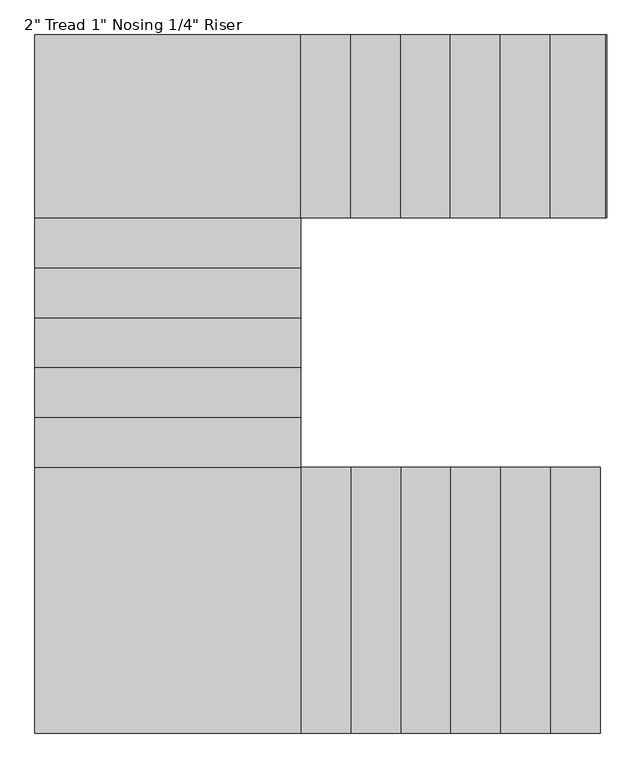
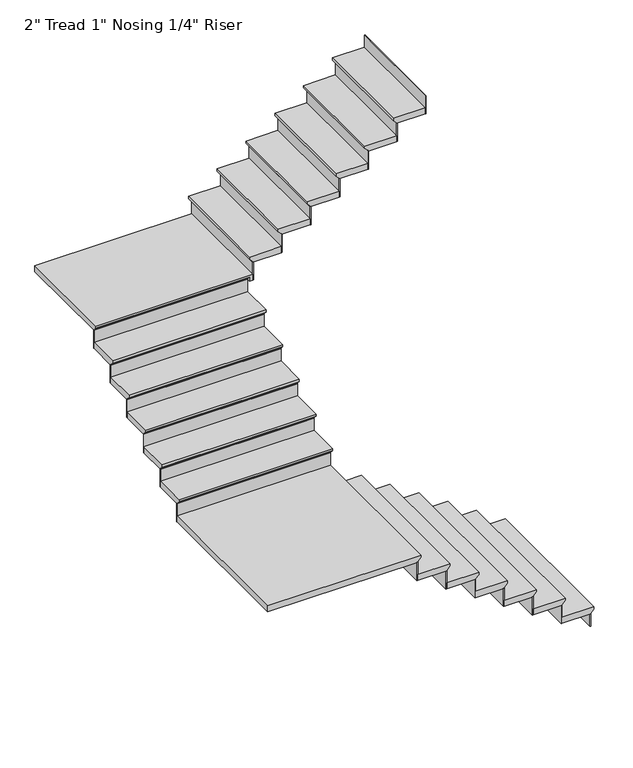
"""IFC4 building model written with IfcOpenShell, lengths in millimetres: stair flight geometry."""

from ifc_helpers import new_model, si_unit, origin, place, context, project, spatial, faceted_brep, source, transform, mapped, element, save


def stair_flight_e1114729(model_context):
    return source(origin(), model_context, "Body", "Brep", [
        faceted_brep([(-2515.2117403, -5163.0426559, 12782.55), (-2515.2117403, -5163.0426559, 12801.6), (-2515.2117403, -6382.2426559, 12801.6), (-2515.2117403, -6382.2426559, 12782.55), (-2540.6117403, -5163.0426559, 12757.15), (-2540.6117403, -6382.2426559, 12757.15), (-2769.2117403, -5163.0426559, 12801.6), (-2769.2117403, -6382.2426559, 12801.6), (-2540.6117403, -6382.2426559, 12750.8), (-2769.2117403, -6382.2426559, 12750.8), (-2769.2117403, -5163.0426559, 12750.8), (-2540.6117403, -5163.0426559, 12750.8)], [[[0, 1, 2, 3]], [[4, 0, 3, 5]], [[2, 1, 6, 7]], [[8, 9, 10, 11]], [[2, 7, 9, 8, 5, 3]], [[8, 11, 4, 5]], [[6, 1, 0, 4, 11, 10]], [[7, 6, 10, 9]]]),
        faceted_brep([(-2540.6117403, -5163.0426559, 12750.8), (-2540.6117403, -5163.0426559, 12649.2), (-2546.9617403, -5163.0426559, 12649.2), (-2546.9617403, -5163.0426559, 12750.8), (-2540.6117403, -6382.2426559, 12750.8), (-2546.9617403, -6382.2426559, 12750.8), (-2546.9617403, -6382.2426559, 12649.2), (-2540.6117403, -6382.2426559, 12649.2)], [[[0, 1, 2, 3]], [[4, 5, 6, 7]], [[1, 0, 4, 7]], [[2, 1, 7, 6]], [[3, 2, 6, 5]], [[0, 3, 5, 4]]]),
        faceted_brep([(-2769.2117403, -5163.0426559, 12903.2), (-2769.2117403, -5163.0426559, 12750.8), (-2775.5617403, -5163.0426559, 12750.8), (-2775.5617403, -5163.0426559, 12903.2), (-2769.2117403, -6382.2426559, 12903.2), (-2775.5617403, -6382.2426559, 12903.2), (-2775.5617403, -6382.2426559, 12750.8), (-2769.2117403, -6382.2426559, 12750.8)], [[[0, 1, 2, 3]], [[4, 5, 6, 7]], [[1, 0, 4, 7]], [[2, 1, 7, 6]], [[3, 2, 6, 5]], [[0, 3, 5, 4]]]),
        faceted_brep([(-2743.8117403, -6382.2426559, 12954.0), (-2743.8117403, -5163.0426559, 12954.0), (-2997.8117403, -5163.0426559, 12954.0), (-2997.8117403, -6382.2426559, 12954.0), (-2769.2117403, -6382.2426559, 12903.2), (-2997.8117403, -6382.2426559, 12903.2), (-2997.8117403, -5163.0426559, 12903.2), (-2769.2117403, -5163.0426559, 12903.2), (-2769.2117403, -6382.2426559, 12909.55), (-2743.8117403, -6382.2426559, 12934.95), (-2769.2117403, -5163.0426559, 12909.55), (-2743.8117403, -5163.0426559, 12934.95)], [[[0, 1, 2, 3]], [[4, 5, 6, 7]], [[0, 3, 5, 4, 8, 9]], [[4, 7, 10, 8]], [[2, 1, 11, 10, 7, 6]], [[3, 2, 6, 5]], [[11, 1, 0, 9]], [[10, 11, 9, 8]]]),
        faceted_brep([(-2997.8117403, -5163.0426559, 13055.6), (-2997.8117403, -5163.0426559, 12903.2), (-3004.1617403, -5163.0426559, 12903.2), (-3004.1617403, -5163.0426559, 13055.6), (-2997.8117403, -6382.2426559, 13055.6), (-3004.1617403, -6382.2426559, 13055.6), (-3004.1617403, -6382.2426559, 12903.2), (-2997.8117403, -6382.2426559, 12903.2)], [[[0, 1, 2, 3]], [[4, 5, 6, 7]], [[1, 0, 4, 7]], [[2, 1, 7, 6]], [[3, 2, 6, 5]], [[0, 3, 5, 4]]]),
        faceted_brep([(-2972.4117403, -6382.2426559, 13106.4), (-2972.4117403, -5163.0426559, 13106.4), (-3226.4117403, -5163.0426559, 13106.4), (-3226.4117403, -6382.2426559, 13106.4), (-2997.8117403, -6382.2426559, 13055.6), (-3226.4117403, -6382.2426559, 13055.6), (-3226.4117403, -5163.0426559, 13055.6), (-2997.8117403, -5163.0426559, 13055.6), (-2997.8117403, -6382.2426559, 13061.95), (-2972.4117403, -6382.2426559, 13087.35), (-2997.8117403, -5163.0426559, 13061.95), (-2972.4117403, -5163.0426559, 13087.35)], [[[0, 1, 2, 3]], [[4, 5, 6, 7]], [[0, 3, 5, 4, 8, 9]], [[4, 7, 10, 8]], [[2, 1, 11, 10, 7, 6]], [[3, 2, 6, 5]], [[11, 1, 0, 9]], [[10, 11, 9, 8]]]),
        faceted_brep([(-3226.4117403, -5163.0426559, 13208.0), (-3226.4117403, -5163.0426559, 13055.6), (-3232.7617403, -5163.0426559, 13055.6), (-3232.7617403, -5163.0426559, 13208.0), (-3226.4117403, -6382.2426559, 13208.0), (-3232.7617403, -6382.2426559, 13208.0), (-3232.7617403, -6382.2426559, 13055.6), (-3226.4117403, -6382.2426559, 13055.6)], [[[0, 1, 2, 3]], [[4, 5, 6, 7]], [[1, 0, 4, 7]], [[2, 1, 7, 6]], [[3, 2, 6, 5]], [[0, 3, 5, 4]]]),
        faceted_brep([(-3201.0117403, -6382.2426559, 13258.8), (-3201.0117403, -5163.0426559, 13258.8), (-3455.0117403, -5163.0426559, 13258.8), (-3455.0117403, -6382.2426559, 13258.8), (-3226.4117403, -6382.2426559, 13208.0), (-3455.0117403, -6382.2426559, 13208.0), (-3455.0117403, -5163.0426559, 13208.0), (-3226.4117403, -5163.0426559, 13208.0), (-3226.4117403, -6382.2426559, 13214.35), (-3201.0117403, -6382.2426559, 13239.75), (-3226.4117403, -5163.0426559, 13214.35), (-3201.0117403, -5163.0426559, 13239.75)], [[[0, 1, 2, 3]], [[4, 5, 6, 7]], [[0, 3, 5, 4, 8, 9]], [[4, 7, 10, 8]], [[2, 1, 11, 10, 7, 6]], [[3, 2, 6, 5]], [[11, 1, 0, 9]], [[10, 11, 9, 8]]]),
        faceted_brep([(-3455.0117403, -5163.0426559, 13360.4), (-3455.0117403, -5163.0426559, 13208.0), (-3461.3617403, -5163.0426559, 13208.0), (-3461.3617403, -5163.0426559, 13360.4), (-3455.0117403, -6382.2426559, 13360.4), (-3461.3617403, -6382.2426559, 13360.4), (-3461.3617403, -6382.2426559, 13208.0), (-3455.0117403, -6382.2426559, 13208.0)], [[[0, 1, 2, 3]], [[4, 5, 6, 7]], [[1, 0, 4, 7]], [[2, 1, 7, 6]], [[3, 2, 6, 5]], [[0, 3, 5, 4]]]),
        faceted_brep([(-3429.6117403, -6382.2426559, 13411.2), (-3429.6117403, -5163.0426559, 13411.2), (-3683.6117403, -5163.0426559, 13411.2), (-3683.6117403, -6382.2426559, 13411.2), (-3455.0117403, -6382.2426559, 13360.4), (-3683.6117403, -6382.2426559, 13360.4), (-3683.6117403, -5163.0426559, 13360.4), (-3455.0117403, -5163.0426559, 13360.4), (-3455.0117403, -6382.2426559, 13366.75), (-3429.6117403, -6382.2426559, 13392.15), (-3455.0117403, -5163.0426559, 13366.75), (-3429.6117403, -5163.0426559, 13392.15)], [[[0, 1, 2, 3]], [[4, 5, 6, 7]], [[0, 3, 5, 4, 8, 9]], [[4, 7, 10, 8]], [[2, 1, 11, 10, 7, 6]], [[3, 2, 6, 5]], [[11, 1, 0, 9]], [[10, 11, 9, 8]]]),
        faceted_brep([(-3683.6117403, -5163.0426559, 13512.8), (-3683.6117403, -5163.0426559, 13360.4), (-3689.9617403, -5163.0426559, 13360.4), (-3689.9617403, -5163.0426559, 13512.8), (-3683.6117403, -6382.2426559, 13512.8), (-3689.9617403, -6382.2426559, 13512.8), (-3689.9617403, -6382.2426559, 13360.4), (-3683.6117403, -6382.2426559, 13360.4)], [[[0, 1, 2, 3]], [[4, 5, 6, 7]], [[1, 0, 4, 7]], [[2, 1, 7, 6]], [[3, 2, 6, 5]], [[0, 3, 5, 4]]]),
        faceted_brep([(-3658.2117403, -6382.2426559, 13563.6), (-3658.2117403, -5163.0426559, 13563.6), (-3912.2117403, -5163.0426559, 13563.6), (-3912.2117403, -6382.2426559, 13563.6), (-3683.6117403, -6382.2426559, 13512.8), (-3912.2117403, -6382.2426559, 13512.8), (-3912.2117403, -5163.0426559, 13512.8), (-3683.6117403, -5163.0426559, 13512.8), (-3683.6117403, -6382.2426559, 13519.15), (-3658.2117403, -6382.2426559, 13544.55), (-3683.6117403, -5163.0426559, 13519.15), (-3658.2117403, -5163.0426559, 13544.55)], [[[0, 1, 2, 3]], [[4, 5, 6, 7]], [[0, 3, 5, 4, 8, 9]], [[4, 7, 10, 8]], [[2, 1, 11, 10, 7, 6]], [[3, 2, 6, 5]], [[11, 1, 0, 9]], [[10, 11, 9, 8]]]),
        faceted_brep([(-3912.2117403, -5163.0426559, 13665.2), (-3912.2117403, -5163.0426559, 13512.8), (-3918.5617403, -5163.0426559, 13512.8), (-3918.5617403, -5163.0426559, 13665.2), (-3912.2117403, -6382.2426559, 13665.2), (-3918.5617403, -6382.2426559, 13665.2), (-3918.5617403, -6382.2426559, 13512.8), (-3912.2117403, -6382.2426559, 13512.8)], [[[0, 1, 2, 3]], [[4, 5, 6, 7]], [[1, 0, 4, 7]], [[2, 1, 7, 6]], [[3, 2, 6, 5]], [[0, 3, 5, 4]]]),
        faceted_brep([(-5106.0117403, -5137.6426559, 13716.0), (-5106.0117403, -6382.2426559, 13716.0), (-3886.8117403, -6382.2426559, 13716.0), (-3886.8117403, -5137.6426559, 13716.0), (-5106.0117403, -6382.2426559, 13665.2), (-5106.0117403, -5137.6426559, 13665.2), (-3886.8117403, -5137.6426559, 13665.2), (-3886.8117403, -5163.0426559, 13665.2), (-3912.2117403, -5163.0426559, 13665.2), (-3912.2117403, -6382.2426559, 13665.2), (-3912.2117403, -6382.2426559, 13671.55), (-3886.8117403, -6382.2426559, 13696.95), (-3912.2117403, -5163.0426559, 13671.55), (-3886.8117403, -5163.0426559, 13696.95)], [[[0, 1, 2, 3]], [[4, 5, 6, 7, 8, 9]], [[1, 0, 5, 4]], [[2, 1, 4, 9, 10, 11]], [[9, 8, 12, 10]], [[8, 7, 13, 12]], [[3, 2, 11, 13, 7, 6]], [[0, 3, 6, 5]], [[11, 10, 12, 13]]]),
        faceted_brep([(-3886.8117403, -5137.6426559, 13817.6), (-3886.8117403, -5137.6426559, 13665.2), (-3886.8117403, -5131.2926559, 13665.2), (-3886.8117403, -5131.2926559, 13817.6), (-5106.0117403, -5137.6426559, 13817.6), (-5106.0117403, -5131.2926559, 13817.6), (-5106.0117403, -5131.2926559, 13665.2), (-5106.0117403, -5137.6426559, 13665.2)], [[[0, 1, 2, 3]], [[4, 5, 6, 7]], [[1, 0, 4, 7]], [[2, 1, 7, 6]], [[3, 2, 6, 5]], [[0, 3, 5, 4]]]),
        faceted_brep([(-5106.0117403, -5163.0426559, 13868.4), (-3886.8117403, -5163.0426559, 13868.4), (-3886.8117403, -4909.0426559, 13868.4), (-5106.0117403, -4909.0426559, 13868.4), (-5106.0117403, -5137.6426559, 13817.6), (-5106.0117403, -4909.0426559, 13817.6), (-3886.8117403, -4909.0426559, 13817.6), (-3886.8117403, -5137.6426559, 13817.6), (-5106.0117403, -5137.6426559, 13823.95), (-5106.0117403, -5163.0426559, 13849.35), (-3886.8117403, -5137.6426559, 13823.95), (-3886.8117403, -5163.0426559, 13849.35)], [[[0, 1, 2, 3]], [[4, 5, 6, 7]], [[0, 3, 5, 4, 8, 9]], [[4, 7, 10, 8]], [[2, 1, 11, 10, 7, 6]], [[3, 2, 6, 5]], [[11, 1, 0, 9]], [[10, 11, 9, 8]]]),
        faceted_brep([(-3886.8117403, -4909.0426559, 13970.0), (-3886.8117403, -4909.0426559, 13817.6), (-3886.8117403, -4902.6926559, 13817.6), (-3886.8117403, -4902.6926559, 13970.0), (-5106.0117403, -4909.0426559, 13970.0), (-5106.0117403, -4902.6926559, 13970.0), (-5106.0117403, -4902.6926559, 13817.6), (-5106.0117403, -4909.0426559, 13817.6)], [[[0, 1, 2, 3]], [[4, 5, 6, 7]], [[1, 0, 4, 7]], [[2, 1, 7, 6]], [[3, 2, 6, 5]], [[0, 3, 5, 4]]]),
        faceted_brep([(-5106.0117403, -4934.4426559, 14020.8), (-3886.8117403, -4934.4426559, 14020.8), (-3886.8117403, -4680.4426559, 14020.8), (-5106.0117403, -4680.4426559, 14020.8), (-5106.0117403, -4909.0426559, 13970.0), (-5106.0117403, -4680.4426559, 13970.0), (-3886.8117403, -4680.4426559, 13970.0), (-3886.8117403, -4909.0426559, 13970.0), (-5106.0117403, -4909.0426559, 13976.35), (-5106.0117403, -4934.4426559, 14001.75), (-3886.8117403, -4909.0426559, 13976.35), (-3886.8117403, -4934.4426559, 14001.75)], [[[0, 1, 2, 3]], [[4, 5, 6, 7]], [[0, 3, 5, 4, 8, 9]], [[4, 7, 10, 8]], [[2, 1, 11, 10, 7, 6]], [[3, 2, 6, 5]], [[11, 1, 0, 9]], [[10, 11, 9, 8]]]),
        faceted_brep([(-3886.8117403, -4680.4426559, 14122.4), (-3886.8117403, -4680.4426559, 13970.0), (-3886.8117403, -4674.0926559, 13970.0), (-3886.8117403, -4674.0926559, 14122.4), (-5106.0117403, -4680.4426559, 14122.4), (-5106.0117403, -4674.0926559, 14122.4), (-5106.0117403, -4674.0926559, 13970.0), (-5106.0117403, -4680.4426559, 13970.0)], [[[0, 1, 2, 3]], [[4, 5, 6, 7]], [[1, 0, 4, 7]], [[2, 1, 7, 6]], [[3, 2, 6, 5]], [[0, 3, 5, 4]]]),
        faceted_brep([(-5106.0117403, -4705.8426559, 14173.2), (-3886.8117403, -4705.8426559, 14173.2), (-3886.8117403, -4451.8426559, 14173.2), (-5106.0117403, -4451.8426559, 14173.2), (-5106.0117403, -4680.4426559, 14122.4), (-5106.0117403, -4451.8426559, 14122.4), (-3886.8117403, -4451.8426559, 14122.4), (-3886.8117403, -4680.4426559, 14122.4), (-5106.0117403, -4680.4426559, 14128.75), (-5106.0117403, -4705.8426559, 14154.15), (-3886.8117403, -4680.4426559, 14128.75), (-3886.8117403, -4705.8426559, 14154.15)], [[[0, 1, 2, 3]], [[4, 5, 6, 7]], [[0, 3, 5, 4, 8, 9]], [[4, 7, 10, 8]], [[2, 1, 11, 10, 7, 6]], [[3, 2, 6, 5]], [[11, 1, 0, 9]], [[10, 11, 9, 8]]]),
        faceted_brep([(-3886.8117403, -4451.8426559, 14274.8), (-3886.8117403, -4451.8426559, 14122.4), (-3886.8117403, -4445.4926559, 14122.4), (-3886.8117403, -4445.4926559, 14274.8), (-5106.0117403, -4451.8426559, 14274.8), (-5106.0117403, -4445.4926559, 14274.8), (-5106.0117403, -4445.4926559, 14122.4), (-5106.0117403, -4451.8426559, 14122.4)], [[[0, 1, 2, 3]], [[4, 5, 6, 7]], [[1, 0, 4, 7]], [[2, 1, 7, 6]], [[3, 2, 6, 5]], [[0, 3, 5, 4]]]),
        faceted_brep([(-5106.0117403, -4477.2426559, 14325.6), (-3886.8117403, -4477.2426559, 14325.6), (-3886.8117403, -4223.2426559, 14325.6), (-5106.0117403, -4223.2426559, 14325.6), (-5106.0117403, -4451.8426559, 14274.8), (-5106.0117403, -4223.2426559, 14274.8), (-3886.8117403, -4223.2426559, 14274.8), (-3886.8117403, -4451.8426559, 14274.8), (-5106.0117403, -4451.8426559, 14281.15), (-5106.0117403, -4477.2426559, 14306.55), (-3886.8117403, -4451.8426559, 14281.15), (-3886.8117403, -4477.2426559, 14306.55)], [[[0, 1, 2, 3]], [[4, 5, 6, 7]], [[0, 3, 5, 4, 8, 9]], [[4, 7, 10, 8]], [[2, 1, 11, 10, 7, 6]], [[3, 2, 6, 5]], [[11, 1, 0, 9]], [[10, 11, 9, 8]]]),
        faceted_brep([(-3886.8117403, -4223.2426559, 14427.2), (-3886.8117403, -4223.2426559, 14274.8), (-3886.8117403, -4216.8926559, 14274.8), (-3886.8117403, -4216.8926559, 14427.2), (-5106.0117403, -4223.2426559, 14427.2), (-5106.0117403, -4216.8926559, 14427.2), (-5106.0117403, -4216.8926559, 14274.8), (-5106.0117403, -4223.2426559, 14274.8)], [[[0, 1, 2, 3]], [[4, 5, 6, 7]], [[1, 0, 4, 7]], [[2, 1, 7, 6]], [[3, 2, 6, 5]], [[0, 3, 5, 4]]]),
        faceted_brep([(-5106.0117403, -4248.6426559, 14478.0), (-3886.8117403, -4248.6426559, 14478.0), (-3886.8117403, -3994.6426559, 14478.0), (-5106.0117403, -3994.6426559, 14478.0), (-5106.0117403, -4223.2426559, 14427.2), (-5106.0117403, -3994.6426559, 14427.2), (-3886.8117403, -3994.6426559, 14427.2), (-3886.8117403, -4223.2426559, 14427.2), (-5106.0117403, -4223.2426559, 14433.55), (-5106.0117403, -4248.6426559, 14458.95), (-3886.8117403, -4223.2426559, 14433.55), (-3886.8117403, -4248.6426559, 14458.95)], [[[0, 1, 2, 3]], [[4, 5, 6, 7]], [[0, 3, 5, 4, 8, 9]], [[4, 7, 10, 8]], [[2, 1, 11, 10, 7, 6]], [[3, 2, 6, 5]], [[11, 1, 0, 9]], [[10, 11, 9, 8]]]),
        faceted_brep([(-3886.8117403, -3994.6426559, 14579.6), (-3886.8117403, -3994.6426559, 14427.2), (-3886.8117403, -3988.2926559, 14427.2), (-3886.8117403, -3988.2926559, 14579.6), (-5106.0117403, -3994.6426559, 14579.6), (-5106.0117403, -3988.2926559, 14579.6), (-5106.0117403, -3988.2926559, 14427.2), (-5106.0117403, -3994.6426559, 14427.2)], [[[0, 1, 2, 3]], [[4, 5, 6, 7]], [[1, 0, 4, 7]], [[2, 1, 7, 6]], [[3, 2, 6, 5]], [[0, 3, 5, 4]]]),
        faceted_brep([(-3861.4117403, -3181.8426559, 14630.4), (-5106.0117403, -3181.8426559, 14630.4), (-5106.0117403, -4020.0426559, 14630.4), (-3861.4117403, -4020.0426559, 14630.4), (-5106.0117403, -3181.8426559, 14579.6), (-3861.4117403, -3181.8426559, 14579.6), (-3861.4117403, -4020.0426559, 14579.6), (-3886.8117403, -4020.0426559, 14579.6), (-3886.8117403, -3994.6426559, 14579.6), (-5106.0117403, -3994.6426559, 14579.6), (-5106.0117403, -3994.6426559, 14585.95), (-5106.0117403, -4020.0426559, 14611.35), (-3886.8117403, -3994.6426559, 14585.95), (-3886.8117403, -4020.0426559, 14611.35)], [[[0, 1, 2, 3]], [[4, 5, 6, 7, 8, 9]], [[1, 0, 5, 4]], [[2, 1, 4, 9, 10, 11]], [[9, 8, 12, 10]], [[8, 7, 13, 12]], [[3, 2, 11, 13, 7, 6]], [[0, 3, 6, 5]], [[11, 10, 12, 13]]]),
        faceted_brep([(-3861.4117403, -4020.0426559, 14732.0), (-3861.4117403, -4020.0426559, 14579.6), (-3855.0617403, -4020.0426559, 14579.6), (-3855.0617403, -4020.0426559, 14732.0), (-3861.4117403, -3181.8426559, 14732.0), (-3855.0617403, -3181.8426559, 14732.0), (-3855.0617403, -3181.8426559, 14579.6), (-3861.4117403, -3181.8426559, 14579.6)], [[[0, 1, 2, 3]], [[4, 5, 6, 7]], [[1, 0, 4, 7]], [[2, 1, 7, 6]], [[3, 2, 6, 5]], [[0, 3, 5, 4]]]),
        faceted_brep([(-3886.8117403, -3181.8426559, 14782.8), (-3886.8117403, -4020.0426559, 14782.8), (-3632.8117403, -4020.0426559, 14782.8), (-3632.8117403, -3181.8426559, 14782.8), (-3861.4117403, -3181.8426559, 14732.0), (-3632.8117403, -3181.8426559, 14732.0), (-3632.8117403, -4020.0426559, 14732.0), (-3861.4117403, -4020.0426559, 14732.0), (-3861.4117403, -3181.8426559, 14738.35), (-3886.8117403, -3181.8426559, 14763.75), (-3861.4117403, -4020.0426559, 14738.35), (-3886.8117403, -4020.0426559, 14763.75)], [[[0, 1, 2, 3]], [[4, 5, 6, 7]], [[0, 3, 5, 4, 8, 9]], [[4, 7, 10, 8]], [[2, 1, 11, 10, 7, 6]], [[3, 2, 6, 5]], [[11, 1, 0, 9]], [[10, 11, 9, 8]]]),
        faceted_brep([(-3632.8117403, -4020.0426559, 14884.4), (-3632.8117403, -4020.0426559, 14732.0), (-3626.4617403, -4020.0426559, 14732.0), (-3626.4617403, -4020.0426559, 14884.4), (-3632.8117403, -3181.8426559, 14884.4), (-3626.4617403, -3181.8426559, 14884.4), (-3626.4617403, -3181.8426559, 14732.0), (-3632.8117403, -3181.8426559, 14732.0)], [[[0, 1, 2, 3]], [[4, 5, 6, 7]], [[1, 0, 4, 7]], [[2, 1, 7, 6]], [[3, 2, 6, 5]], [[0, 3, 5, 4]]]),
        faceted_brep([(-3658.2117403, -3181.8426559, 14935.2), (-3658.2117403, -4020.0426559, 14935.2), (-3404.2117403, -4020.0426559, 14935.2), (-3404.2117403, -3181.8426559, 14935.2), (-3632.8117403, -3181.8426559, 14884.4), (-3404.2117403, -3181.8426559, 14884.4), (-3404.2117403, -4020.0426559, 14884.4), (-3632.8117403, -4020.0426559, 14884.4), (-3632.8117403, -3181.8426559, 14890.75), (-3658.2117403, -3181.8426559, 14916.15), (-3632.8117403, -4020.0426559, 14890.75), (-3658.2117403, -4020.0426559, 14916.15)], [[[0, 1, 2, 3]], [[4, 5, 6, 7]], [[0, 3, 5, 4, 8, 9]], [[4, 7, 10, 8]], [[2, 1, 11, 10, 7, 6]], [[3, 2, 6, 5]], [[11, 1, 0, 9]], [[10, 11, 9, 8]]]),
        faceted_brep([(-3404.2117403, -4020.0426559, 15036.8), (-3404.2117403, -4020.0426559, 14884.4), (-3397.8617403, -4020.0426559, 14884.4), (-3397.8617403, -4020.0426559, 15036.8), (-3404.2117403, -3181.8426559, 15036.8), (-3397.8617403, -3181.8426559, 15036.8), (-3397.8617403, -3181.8426559, 14884.4), (-3404.2117403, -3181.8426559, 14884.4)], [[[0, 1, 2, 3]], [[4, 5, 6, 7]], [[1, 0, 4, 7]], [[2, 1, 7, 6]], [[3, 2, 6, 5]], [[0, 3, 5, 4]]]),
        faceted_brep([(-3429.6117403, -3181.8426559, 15087.6), (-3429.6117403, -4020.0426559, 15087.6), (-3175.6117403, -4020.0426559, 15087.6), (-3175.6117403, -3181.8426559, 15087.6), (-3404.2117403, -3181.8426559, 15036.8), (-3175.6117403, -3181.8426559, 15036.8), (-3175.6117403, -4020.0426559, 15036.8), (-3404.2117403, -4020.0426559, 15036.8), (-3404.2117403, -3181.8426559, 15043.15), (-3429.6117403, -3181.8426559, 15068.55), (-3404.2117403, -4020.0426559, 15043.15), (-3429.6117403, -4020.0426559, 15068.55)], [[[0, 1, 2, 3]], [[4, 5, 6, 7]], [[0, 3, 5, 4, 8, 9]], [[4, 7, 10, 8]], [[2, 1, 11, 10, 7, 6]], [[3, 2, 6, 5]], [[11, 1, 0, 9]], [[10, 11, 9, 8]]]),
        faceted_brep([(-3175.6117403, -4020.0426559, 15189.2), (-3175.6117403, -4020.0426559, 15036.8), (-3169.2617403, -4020.0426559, 15036.8), (-3169.2617403, -4020.0426559, 15189.2), (-3175.6117403, -3181.8426559, 15189.2), (-3169.2617403, -3181.8426559, 15189.2), (-3169.2617403, -3181.8426559, 15036.8), (-3175.6117403, -3181.8426559, 15036.8)], [[[0, 1, 2, 3]], [[4, 5, 6, 7]], [[1, 0, 4, 7]], [[2, 1, 7, 6]], [[3, 2, 6, 5]], [[0, 3, 5, 4]]]),
        faceted_brep([(-3201.0117403, -3181.8426559, 15240.0), (-3201.0117403, -4020.0426559, 15240.0), (-2947.0117403, -4020.0426559, 15240.0), (-2947.0117403, -3181.8426559, 15240.0), (-3175.6117403, -3181.8426559, 15189.2), (-2947.0117403, -3181.8426559, 15189.2), (-2947.0117403, -4020.0426559, 15189.2), (-3175.6117403, -4020.0426559, 15189.2), (-3175.6117403, -3181.8426559, 15195.55), (-3201.0117403, -3181.8426559, 15220.95), (-3175.6117403, -4020.0426559, 15195.55), (-3201.0117403, -4020.0426559, 15220.95)], [[[0, 1, 2, 3]], [[4, 5, 6, 7]], [[0, 3, 5, 4, 8, 9]], [[4, 7, 10, 8]], [[2, 1, 11, 10, 7, 6]], [[3, 2, 6, 5]], [[11, 1, 0, 9]], [[10, 11, 9, 8]]]),
        faceted_brep([(-2947.0117403, -4020.0426559, 15341.6), (-2947.0117403, -4020.0426559, 15189.2), (-2940.6617403, -4020.0426559, 15189.2), (-2940.6617403, -4020.0426559, 15341.6), (-2947.0117403, -3181.8426559, 15341.6), (-2940.6617403, -3181.8426559, 15341.6), (-2940.6617403, -3181.8426559, 15189.2), (-2947.0117403, -3181.8426559, 15189.2)], [[[0, 1, 2, 3]], [[4, 5, 6, 7]], [[1, 0, 4, 7]], [[2, 1, 7, 6]], [[3, 2, 6, 5]], [[0, 3, 5, 4]]]),
        faceted_brep([(-2972.4117403, -3181.8426559, 15392.4), (-2972.4117403, -4020.0426559, 15392.4), (-2718.4117403, -4020.0426559, 15392.4), (-2718.4117403, -3181.8426559, 15392.4), (-2947.0117403, -3181.8426559, 15341.6), (-2718.4117403, -3181.8426559, 15341.6), (-2718.4117403, -4020.0426559, 15341.6), (-2947.0117403, -4020.0426559, 15341.6), (-2947.0117403, -3181.8426559, 15347.95), (-2972.4117403, -3181.8426559, 15373.35), (-2947.0117403, -4020.0426559, 15347.95), (-2972.4117403, -4020.0426559, 15373.35)], [[[0, 1, 2, 3]], [[4, 5, 6, 7]], [[0, 3, 5, 4, 8, 9]], [[4, 7, 10, 8]], [[2, 1, 11, 10, 7, 6]], [[3, 2, 6, 5]], [[11, 1, 0, 9]], [[10, 11, 9, 8]]]),
        faceted_brep([(-2718.4117403, -4020.0426559, 15494.0), (-2718.4117403, -4020.0426559, 15341.6), (-2712.0617403, -4020.0426559, 15341.6), (-2712.0617403, -4020.0426559, 15494.0), (-2718.4117403, -3181.8426559, 15494.0), (-2712.0617403, -3181.8426559, 15494.0), (-2712.0617403, -3181.8426559, 15341.6), (-2718.4117403, -3181.8426559, 15341.6)], [[[0, 1, 2, 3]], [[4, 5, 6, 7]], [[1, 0, 4, 7]], [[2, 1, 7, 6]], [[3, 2, 6, 5]], [[0, 3, 5, 4]]]),
        faceted_brep([(-2489.8117403, -4020.0426559, 15646.4), (-2489.8117403, -4020.0426559, 15494.0), (-2483.4617403, -4020.0426559, 15494.0), (-2483.4617403, -4020.0426559, 15646.4), (-2489.8117403, -3181.8426559, 15646.4), (-2483.4617403, -3181.8426559, 15646.4), (-2483.4617403, -3181.8426559, 15494.0), (-2489.8117403, -3181.8426559, 15494.0)], [[[0, 1, 2, 3]], [[4, 5, 6, 7]], [[1, 0, 4, 7]], [[2, 1, 7, 6]], [[3, 2, 6, 5]], [[0, 3, 5, 4]]]),
        faceted_brep([(-2743.8117403, -3181.8426559, 15544.8), (-2743.8117403, -4020.0426559, 15544.8), (-2489.8117403, -4020.0426559, 15544.8), (-2489.8117403, -3181.8426559, 15544.8), (-2718.4117403, -3181.8426559, 15494.0), (-2489.8117403, -3181.8426559, 15494.0), (-2489.8117403, -4020.0426559, 15494.0), (-2718.4117403, -4020.0426559, 15494.0), (-2718.4117403, -3181.8426559, 15500.35), (-2743.8117403, -3181.8426559, 15525.75), (-2718.4117403, -4020.0426559, 15500.35), (-2743.8117403, -4020.0426559, 15525.75)], [[[0, 1, 2, 3]], [[4, 5, 6, 7]], [[0, 3, 5, 4, 8, 9]], [[4, 7, 10, 8]], [[2, 1, 11, 10, 7, 6]], [[3, 2, 6, 5]], [[11, 1, 0, 9]], [[10, 11, 9, 8]]]),
    ])


if __name__ == "__main__":
    model = new_model("IFC4")
    model_context = context("Model", 3, world=origin())
    ifc_project = project(units=[si_unit("LENGTHUNIT", "METRE", prefix="MILLI")], contexts=[model_context])
    site = spatial("IfcSite", under=ifc_project)
    building = spatial("IfcBuilding", under=site)
    placement = place(None, origin())
    stair_flight_shape = stair_flight_e1114729(model_context)
    element("IfcStairFlight", 1, ObjectType="2\" Tread 1\" Nosing 1/4\" Riser", at=placement, inside=building, context=model_context, shape_type="MappedRepresentation", body=[
        mapped(stair_flight_shape, transform((0.0, 0.0, 0.0), x_axis=(1.0, 0.0, 0.0), y_axis=(0.0, 1.0, 0.0), z_axis=(0.0, 0.0, 1.0))),
    ])
    save(model, "model.ifc")

# Revit data of these elements
# Element 1 (IfcStairFlight, "2\" Tread 1\" Nosing 1/4\" Riser")
#   Materials on its faces: "Wood Planks"
# Materials
#   "Wood Planks": class "Wood", colour RGB 193 160 115, transparency 0, Description = "Physical material.", Cost = 0
